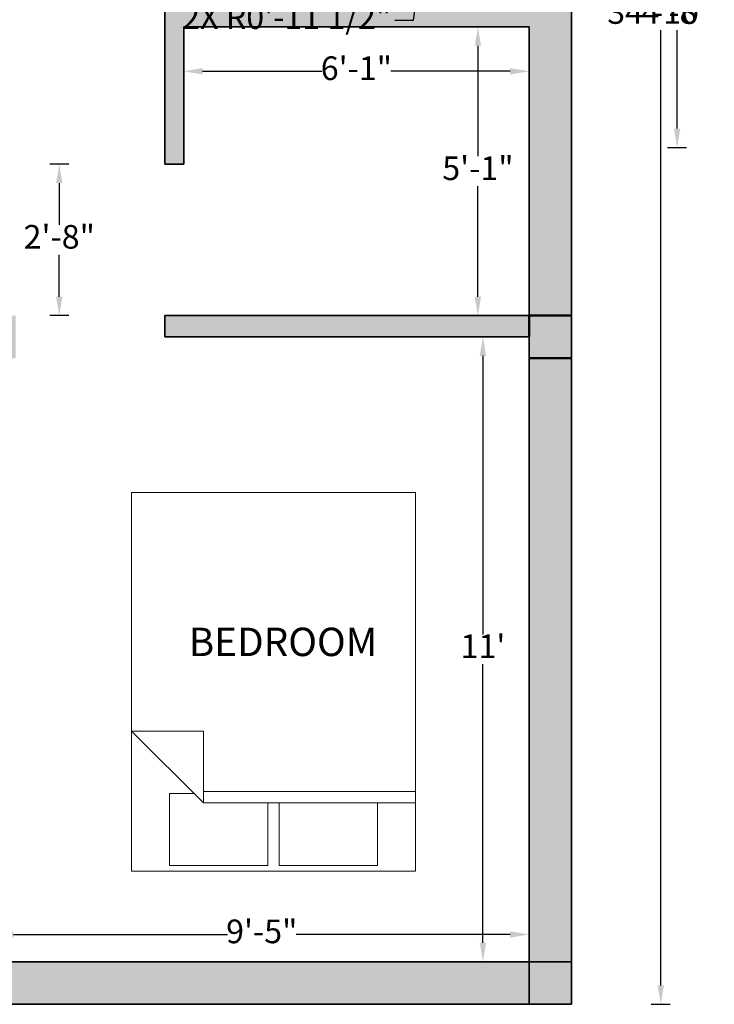
# Model space of a CAD drawing. Units: inches. Extents: x 2244 to 2676, y 593 to 1067.
# Tile 2 of 4: x 2530 to 2676, y 623 to 831. Entities that reach past the tile are written whole.
import ezdxf

# ---------------------------------------------------------------- set-up
doc = ezdxf.new("R2010")
doc.units = ezdxf.units.IN
for name, color, linetype, lineweight in [('A-ANNO-DIMS', 2, 'Continuous', 18), ('A-AREA-IDEN', 7, 'Continuous', 25), ('A-COLS', 7, 'Continuous', 50), ('A-COLS-PATT', 1, 'Continuous', 13), ('A-FURN', 8, 'Continuous', 18), ('A-WALL', 7, 'Continuous', 35)]:
    doc.layers.add(name, color=color, linetype=linetype, lineweight=lineweight)
doc.layers.add('A-WALL-PATT', color=159, linetype='Continuous', lineweight=13, true_color=0x22346e)
doc.styles.get("Standard").update_dxf_attribs({"font": 'arial.ttf'})
doc.dimstyles.new('ISO-25', dxfattribs={"dimtxt": 5, "dimasz": 4, "dimexe": 2, "dimexo": 2, "dimtad": 0, "dimtih": 1, "dimtoh": 1, "dimlunit": 3, "dimtxsty": 'Standard', "dimcen": 2.5, "dimadec": 0, "dimazin": 0, "dimtfac": 1, "dimtmove": 0, "dimatfit": 3, "dimfxl": 2, "dimfxlon": 1, "dimarcsym": 0})

# ---------------------------------------------------------------- blocks, each defined once
blk = doc.blocks.new('*D12')
at = {"layer": 'A-ANNO-DIMS', "color": 0, "lineweight": -2, "transparency": 16777216}
for p, q in [((2628.39, 829.42), (2624.39, 829.42)), ((2626.39, 825.42), (2626.39, 802.1)), ((2626.39, 772.42), (2626.39, 795.74)), ((2628.39, 768.42), (2624.39, 768.42))]:
    blk.add_line(p, q, dxfattribs=at)
at = {"layer": 'A-ANNO-DIMS', "color": 0, "transparency": 16777216}
for points in [[(2625.72, 825.42), (2627.05, 825.42), (2626.39, 829.42)], [(2625.72, 772.42), (2627.05, 772.42), (2626.39, 768.42)]]:
    blk.add_solid(points, dxfattribs=at)
at = {"layer": 'Defpoints', "color": 0, "transparency": 16777216}
for p in [(2637.2, 829.42), (2626.39, 768.42), (2637.2, 768.42)]:
    blk.add_point(p, dxfattribs=at)
at = {"layer": 'A-ANNO-DIMS', "color": 0, "transparency": 16777216, "insert": (2626.39, 798.92), "char_height": 5, "attachment_point": 5}
blk.add_mtext('5\'-1"', dxfattribs=at)
blk = doc.blocks.new('*D13')
at = {"layer": 'A-ANNO-DIMS', "color": 0, "lineweight": -2, "transparency": 16777216}
for p, q in [((2564.2, 822.04), (2564.2, 818.04)), ((2637.2, 822.04), (2637.2, 818.04)), ((2568.2, 820.04), (2593.41, 820.04)), ((2633.2, 820.04), (2607.98, 820.04))]:
    blk.add_line(p, q, dxfattribs=at)
at = {"layer": 'A-ANNO-DIMS', "color": 0, "transparency": 16777216}
for points in [[(2568.2, 820.71), (2568.2, 819.37), (2564.2, 820.04)], [(2633.2, 820.71), (2633.2, 819.37), (2637.2, 820.04)]]:
    blk.add_solid(points, dxfattribs=at)
at = {"layer": 'Defpoints', "color": 0, "transparency": 16777216}
for p in [(2564.2, 829.42), (2637.2, 829.42), (2637.2, 820.04)]:
    blk.add_point(p, dxfattribs=at)
at = {"layer": 'A-ANNO-DIMS', "color": 0, "transparency": 16777216, "insert": (2600.7, 820.04), "char_height": 5, "attachment_point": 5}
blk.add_mtext('6\'-1"', dxfattribs=at)
blk = doc.blocks.new('*D14')
at = {"layer": 'A-ANNO-DIMS', "color": 0, "lineweight": -2, "transparency": 16777216}
for p, q in [((2629.45, 763.92), (2625.45, 763.92)), ((2627.45, 759.92), (2627.45, 701.06)), ((2627.45, 635.92), (2627.45, 694.79)), ((2629.45, 631.92), (2625.45, 631.92))]:
    blk.add_line(p, q, dxfattribs=at)
at = {"layer": 'A-ANNO-DIMS', "color": 0, "transparency": 16777216}
for points in [[(2626.78, 759.92), (2628.12, 759.92), (2627.45, 763.92)], [(2626.78, 635.92), (2628.12, 635.92), (2627.45, 631.92)]]:
    blk.add_solid(points, dxfattribs=at)
at = {"layer": 'Defpoints', "color": 0, "transparency": 16777216}
for p in [(2637.2, 763.92), (2627.45, 631.92), (2637.2, 631.92)]:
    blk.add_point(p, dxfattribs=at)
at = {"layer": 'A-ANNO-DIMS', "color": 0, "transparency": 16777216, "insert": (2627.45, 697.92), "char_height": 5, "attachment_point": 5}
blk.add_mtext("11'", dxfattribs=at)
blk = doc.blocks.new('*D15')
at = {"layer": 'A-ANNO-DIMS', "color": 0, "lineweight": -2, "transparency": 16777216}
for p, q in [((2524.2, 639.68), (2524.2, 635.68)), ((2637.2, 639.68), (2637.2, 635.68)), ((2528.2, 637.68), (2573.43, 637.68)), ((2633.2, 637.68), (2587.97, 637.68))]:
    blk.add_line(p, q, dxfattribs=at)
at = {"layer": 'A-ANNO-DIMS', "color": 0, "transparency": 16777216}
for points in [[(2528.2, 638.34), (2528.2, 637.01), (2524.2, 637.68)], [(2633.2, 638.34), (2633.2, 637.01), (2637.2, 637.68)]]:
    blk.add_solid(points, dxfattribs=at)
at = {"layer": 'Defpoints', "color": 0, "transparency": 16777216}
for p in [(2524.2, 645.95), (2637.2, 645.95), (2637.2, 637.68)]:
    blk.add_point(p, dxfattribs=at)
at = {"layer": 'A-ANNO-DIMS', "color": 0, "transparency": 16777216, "insert": (2580.7, 637.68), "char_height": 5, "attachment_point": 5}
blk.add_mtext('9\'-5"', dxfattribs=at)
blk = doc.blocks.new('*D22')
at = {"layer": 'A-ANNO-DIMS', "color": 0, "lineweight": -2, "transparency": 16777216}
for p, q in [((2663.04, 1040.92), (2667.04, 1040.92)), ((2665.04, 1036.92), (2665.04, 835.1)), ((2665.04, 626.92), (2665.04, 828.74)), ((2663.04, 622.92), (2667.04, 622.92))]:
    blk.add_line(p, q, dxfattribs=at)
at = {"layer": 'A-ANNO-DIMS', "color": 0, "transparency": 16777216}
for points in [[(2664.38, 1036.92), (2665.71, 1036.92), (2665.04, 1040.92)], [(2664.38, 626.92), (2665.71, 626.92), (2665.04, 622.92)]]:
    blk.add_solid(points, dxfattribs=at)
at = {"layer": 'Defpoints', "color": 0, "transparency": 16777216}
for p in [(2646.2, 1040.92), (2646.2, 622.92), (2665.04, 622.92)]:
    blk.add_point(p, dxfattribs=at)
at = {"layer": 'A-ANNO-DIMS', "color": 0, "transparency": 16777216, "insert": (2665.04, 831.92), "char_height": 5, "attachment_point": 5}
blk.add_mtext('34\'-10"', dxfattribs=at)
blk = doc.blocks.new('Bed - Queen')
for p, q in [((0, -80.00003), (0, 0)), ((0, 0), (59.99999, 0)), ((59.99999, 0), (59.99999, -80.00003)), ((7.99999, -1.2), (28.79998, -1.2)), ((7.99999, -14.4), (7.99999, -1.2)), ((28.79998, -1.2), (28.79998, -14.4)), ((31.19999, -1.2), (51.99999, -1.2)), ((31.19999, -14.4), (31.19999, -1.2)), ((51.99999, -1.2), (51.99999, -16.4)), ((0, -14.4), (44.8, -14.4)), ((59.99999, -29.6), (44.8, -14.4)), ((44.8, -14.4), (44.8, -29.6)), ((51.99999, -16.4), (46.79936, -16.4)), ((44.8, -16.8), (0, -16.8)), ((44.8, -29.6), (59.99999, -29.6)), ((59.99999, -80.00003), (0, -80.00003))]:
    blk.add_line(p, q)
blk = doc.blocks.new('*D42')
at = {"layer": 'A-ANNO-DIMS', "color": 0, "lineweight": -2, "transparency": 16777216}
for p, q in [((2666.5, 859.92), (2670.5, 859.92)), ((2668.5, 855.92), (2668.5, 835.1)), ((2668.5, 807.92), (2668.5, 828.74)), ((2666.5, 803.92), (2670.5, 803.92))]:
    blk.add_line(p, q, dxfattribs=at)
at = {"layer": 'A-ANNO-DIMS', "color": 0, "transparency": 16777216}
for points in [[(2667.83, 855.92), (2669.16, 855.92), (2668.5, 859.92)], [(2667.83, 807.92), (2669.16, 807.92), (2668.5, 803.92)]]:
    blk.add_solid(points, dxfattribs=at)
at = {"layer": 'Defpoints', "color": 0, "transparency": 16777216}
for p in [(2359.7, 859.92), (2668.5, 859.92), (2359.7, 803.92)]:
    blk.add_point(p, dxfattribs=at)
at = {"layer": 'A-ANNO-DIMS', "color": 0, "transparency": 16777216, "insert": (2668.5, 831.92), "char_height": 5, "attachment_point": 5}
blk.add_mtext('4\'-8"', dxfattribs=at)
blk = doc.blocks.new('*D47')
at = {"layer": 'A-ANNO-DIMS', "color": 0, "lineweight": -2, "transparency": 16777216}
for p, q in [((2539.9, 800.42), (2535.9, 800.42)), ((2537.9, 796.42), (2537.9, 787.6)), ((2537.9, 772.42), (2537.9, 781.24)), ((2539.9, 768.42), (2535.9, 768.42))]:
    blk.add_line(p, q, dxfattribs=at)
at = {"layer": 'A-ANNO-DIMS', "color": 0, "transparency": 16777216}
for points in [[(2537.23, 796.42), (2538.56, 796.42), (2537.9, 800.42)], [(2537.23, 772.42), (2538.56, 772.42), (2537.9, 768.42)]]:
    blk.add_solid(points, dxfattribs=at)
at = {"layer": 'Defpoints', "color": 0, "transparency": 16777216}
for p in [(2537.9, 800.42), (2560.2, 800.42), (2560.2, 768.42)]:
    blk.add_point(p, dxfattribs=at)
at = {"layer": 'A-ANNO-DIMS', "color": 0, "transparency": 16777216, "insert": (2537.9, 784.42), "char_height": 5, "attachment_point": 5}
blk.add_mtext('2\'-8"', dxfattribs=at)
blk = doc.blocks.new('*D59')
at = {"layer": 'A-ANNO-DIMS', "color": 0, "lineweight": -2, "transparency": 16777216}
for p, q in [((2615.38, 850), (2613.87, 838.77)), ((2612.8, 830.84), (2613.34, 834.81)), ((2608.8, 830.84), (2612.8, 830.84))]:
    blk.add_line(p, q, dxfattribs=at)
at = {"layer": 'A-ANNO-DIMS', "color": 0, "transparency": 16777216}
blk.add_solid([(2612.68, 834.9), (2614, 834.72), (2613.87, 838.77)], dxfattribs=at)
at = {"layer": 'Defpoints', "color": 0, "transparency": 16777216}
for p in [(2615.38, 850), (2613.87, 838.77)]:
    blk.add_point(p, dxfattribs=at)
at = {"layer": 'A-ANNO-DIMS', "color": 0, "transparency": 16777216, "insert": (2585.96, 830.84), "char_height": 5, "attachment_point": 5}
blk.add_mtext('2X R0\'-11 1/2"', dxfattribs=at)

msp = doc.modelspace()

# ---------------------------------------------------------------- hatches: boundary and pattern name
at = {"layer": 'A-COLS-PATT'}
h = msp.add_hatch(color=256, dxfattribs=at)
h.dxf.hatch_style = 1
h.paths.add_polyline_path([(2285.197, 1040.922), (2276.197, 1040.922), (2276.197, 1031.922), (2285.197, 1031.922)])
h.paths.add_polyline_path([(2402.697, 1040.922), (2393.697, 1040.922), (2393.697, 1031.922), (2398.197, 1031.922), (2402.697, 1031.922)])
h.paths.add_polyline_path([(2528.697, 1040.922), (2519.697, 1040.922), (2519.697, 1031.922), (2524.197, 1031.922), (2528.697, 1031.922)])
h.paths.add_polyline_path([(2646.197, 1040.922), (2637.197, 1040.922), (2637.197, 1031.922), (2646.197, 1031.922)])
h.paths.add_polyline_path([(2646.197, 904.422), (2637.197, 904.422), (2637.197, 899.922), (2637.197, 895.422), (2646.197, 895.422)])
h.paths.add_polyline_path([(2528.697, 904.422), (2519.697, 904.422), (2519.697, 895.422), (2524.197, 895.422), (2528.697, 895.422)])
h.paths.add_polyline_path([(2402.697, 899.922), (2402.697, 904.422), (2393.697, 904.422), (2393.697, 895.422), (2402.697, 895.422)])
h.paths.add_polyline_path([(2285.197, 899.922), (2285.197, 904.422), (2276.197, 904.422), (2276.197, 895.422), (2285.197, 895.422)])
h.paths.add_polyline_path([(2285.197, 768.422), (2276.197, 768.422), (2276.197, 759.422), (2285.197, 759.422), (2285.197, 763.922)])
h.paths.add_polyline_path([(2285.197, 631.922), (2276.197, 631.922), (2276.197, 622.922), (2285.197, 622.922)])
h.paths.add_polyline_path([(2402.697, 631.922), (2398.197, 631.922), (2393.697, 631.922), (2393.697, 622.922), (2402.697, 622.922)])
h.paths.add_polyline_path([(2402.697, 763.922), (2402.697, 768.422), (2398.197, 768.422), (2393.697, 768.422), (2393.697, 759.422), (2402.697, 759.422)])
h.paths.add_polyline_path([(2528.697, 768.422), (2524.197, 768.422), (2519.697, 768.422), (2519.697, 759.422), (2528.697, 759.422)])
h.paths.add_polyline_path([(2528.697, 631.922), (2524.197, 631.922), (2519.697, 631.922), (2519.697, 628.922), (2519.697, 622.922), (2528.697, 622.922)])
h.paths.add_polyline_path([(2646.197, 631.922), (2637.197, 631.922), (2637.197, 622.922), (2646.197, 622.922)])
h.paths.add_polyline_path([(2646.197, 768.422), (2637.197, 768.422), (2637.197, 763.922), (2637.197, 759.422), (2646.197, 759.422)])
at = {"layer": 'A-WALL-PATT'}
h = msp.add_hatch(color=256, dxfattribs=at)
h.dxf.hatch_style = 1
h.paths.add_polyline_path([(2637.197, 1040.922), (2528.697, 1040.922), (2528.697, 1031.922), (2637.197, 1031.922)])
h.paths.add_polyline_path([(2519.697, 1040.922), (2402.697, 1040.922), (2402.697, 1031.922), (2519.697, 1031.922)])
h.paths.add_polyline_path([(2393.697, 1040.922), (2285.197, 1040.922), (2285.197, 1031.922), (2393.697, 1031.922)])
h.paths.add_polyline_path([(2285.197, 1031.922), (2276.197, 1031.922), (2276.197, 904.422), (2285.197, 904.422)])
h.paths.add_polyline_path([(2402.697, 1031.922), (2398.197, 1031.922), (2398.197, 904.422), (2402.697, 904.422)])
h.paths.add_polyline_path([(2483.697, 899.922), (2402.697, 899.922), (2402.697, 895.422), (2483.697, 895.422)])
h.paths.add_polyline_path([(2524.197, 1031.922), (2519.697, 1031.922), (2519.697, 904.422), (2524.197, 904.422)])
h.paths.add_polyline_path([(2637.197, 899.922), (2560.197, 899.922), (2560.197, 895.422), (2637.197, 895.422)])
h.paths.add_polyline_path([(2646.197, 1031.922), (2637.197, 1031.922), (2637.197, 904.422), (2646.197, 904.422)])
h.paths.add_polyline_path([(2646.197, 895.422), (2637.197, 895.422), (2637.197, 834.422), (2564.197, 834.422), (2564.197, 863.422), (2560.197, 863.422), (2560.197, 800.422), (2564.197, 800.422), (2564.197, 829.422), (2637.197, 829.422), (2637.197, 768.422), (2646.197, 768.422)])
h.paths.add_polyline_path([(2646.197, 759.422), (2637.197, 759.422), (2637.197, 631.922), (2646.197, 631.922)])
h.paths.add_polyline_path([(2637.197, 768.422), (2560.197, 768.422), (2560.197, 763.922), (2637.197, 763.922)])
h.paths.add_polyline_path([(2637.197, 631.922), (2528.697, 631.922), (2528.697, 622.922), (2637.197, 622.922)])
h.paths.add_polyline_path([(2524.197, 759.422), (2519.697, 759.422), (2519.697, 631.922), (2524.197, 631.922)])
h.paths.add_polyline_path([(2402.697, 759.422), (2398.197, 759.422), (2398.197, 631.922), (2402.697, 631.922)])
h.paths.add_polyline_path([(2476.697, 768.422), (2402.697, 768.422), (2402.697, 763.922), (2476.697, 763.922)])
h.paths.add_polyline_path([(2459.697, 631.922), (2402.697, 631.922), (2402.697, 622.922), (2459.697, 622.922), (2459.697, 628.922)])
h.paths.add_polyline_path([(2393.697, 631.922), (2285.197, 631.922), (2285.197, 622.922), (2393.697, 622.922)])
h.paths.add_polyline_path([(2285.197, 759.422), (2276.197, 759.422), (2276.197, 631.922), (2285.197, 631.922)])
h.paths.add_polyline_path([(2359.697, 803.922), (2355.197, 803.922), (2355.197, 768.422), (2285.197, 768.422), (2285.197, 763.922), (2359.697, 763.922)])
h.paths.add_polyline_path([(2359.697, 899.922), (2285.197, 899.922), (2285.197, 895.422), (2355.197, 895.422), (2355.197, 859.922), (2359.697, 859.922)])
h.paths.add_polyline_path([(2285.197, 895.422), (2276.197, 895.422), (2276.197, 768.422), (2285.197, 768.422)])

# ---------------------------------------------------------------- linework, layer by layer
at = {"layer": 'A-COLS'}
for p, q in [((2637.197, 768.422), (2637.197, 763.922)), ((2637.197, 768.422), (2646.197, 768.422)), ((2637.197, 759.422), (2646.197, 759.422))]:
    msp.add_line(p, q, dxfattribs=at)
at = {"layer": 'A-WALL'}
for p, q in [((2646.197, 622.922), (2646.197, 1040.922)), ((2560.197, 800.422), (2560.197, 863.422)), ((2564.197, 800.422), (2564.197, 829.422)), ((2637.197, 829.422), (2564.197, 829.422)), ((2637.197, 768.422), (2637.197, 829.422)), ((2564.197, 800.422), (2560.197, 800.422)), ((2637.197, 768.422), (2560.197, 768.422)), ((2560.197, 763.922), (2560.197, 768.422)), ((2637.197, 763.922), (2560.197, 763.922)), ((2637.197, 622.922), (2637.197, 763.922)), ((2524.197, 631.922), (2646.197, 631.922)), ((2276.197, 622.922), (2646.197, 622.922))]:
    msp.add_line(p, q, dxfattribs=at)

# ---------------------------------------------------------------- block references
at = {"layer": 'A-FURN', "rotation": 180}
msp.add_blockref('Bed - Queen', (2613.179, 651.056), dxfattribs=at)

# ---------------------------------------------------------------- texts
at = {"layer": 'A-AREA-IDEN', "insert": (2565.273, 702.494), "char_height": 6, "attachment_point": 1}
msp.add_mtext_dynamic_manual_height_columns('BEDROOM', width=31.51274, gutter_width=12.5, heights=[0], dxfattribs=at)

# ---------------------------------------------------------------- dimensions: what is measured, and where the dimension line sits
at = {"layer": 'A-ANNO-DIMS'}
for base, p1, p2, override, picture, middle in [((2665.043, 622.922), (2646.197, 1040.922), (2646.197, 622.922), {"dimclrd": 0, "dimclre": 0, "dimclrt": 0}, '*D22', (2665.043, 831.922)), ((2668.497, 859.922), (2359.697, 803.922), (2359.697, 859.922), {"dimdec": 1, "dimlfac": 1, "dimrnd": 0, "dimzin": 1, "dimdsep": 46, "dimlunit": 4, "dimfrac": 2}, '*D42', (2668.497, 831.922)), ((2626.387, 768.422), (2637.197, 829.422), (2637.197, 768.422), {"dimclrd": 0, "dimclre": 0, "dimclrt": 0}, '*D12', (2626.387, 798.922)), ((2537.897, 800.422), (2560.197, 768.422), (2560.197, 800.422), {"dimdec": 1, "dimlfac": 1, "dimrnd": 0, "dimzin": 1, "dimdsep": 46, "dimlunit": 4, "dimfrac": 2}, '*D47', (2537.897, 784.422)), ((2627.451, 631.922), (2637.197, 763.922), (2637.197, 631.922), {"dimclrd": 0, "dimclre": 0, "dimclrt": 0}, '*D14', (2627.451, 697.922))]:
    dim = msp.add_linear_dim(base=base, p1=p1, p2=p2, angle=90, dimstyle='ISO-25', override=override, dxfattribs=at)
    dim.commit()
    dim.dimension.update_dxf_attribs({"geometry": picture, "text_midpoint": middle})
dim = msp.add_radius_dim(center=(2615.379, 850.001), mpoint=(2613.87, 838.773), text='2X <>', dimstyle='ISO-25', override={"dimdec": 1, "dimlfac": 1, "dimrnd": 0, "dimzin": 1, "dimdsep": 46, "dimlunit": 4, "dimfrac": 2}, dxfattribs=at)
dim.commit()
dim.dimension.update_dxf_attribs({"geometry": '*D59', "text_midpoint": (2585.959, 830.844)})
for base, p1, p2, picture, middle in [((2637.197, 820.041), (2564.197, 829.422), (2637.197, 829.422), '*D13', (2600.697, 820.041)), ((2637.197, 637.678), (2524.197, 645.948), (2637.197, 645.948), '*D15', (2580.697, 637.678))]:
    dim = msp.add_linear_dim(base=base, p1=p1, p2=p2, dimstyle='ISO-25', override={"dimclrd": 0, "dimclre": 0, "dimclrt": 0}, dxfattribs=at)
    dim.commit()
    dim.dimension.update_dxf_attribs({"geometry": picture, "text_midpoint": middle})

doc.saveas('drawing.dxf')
